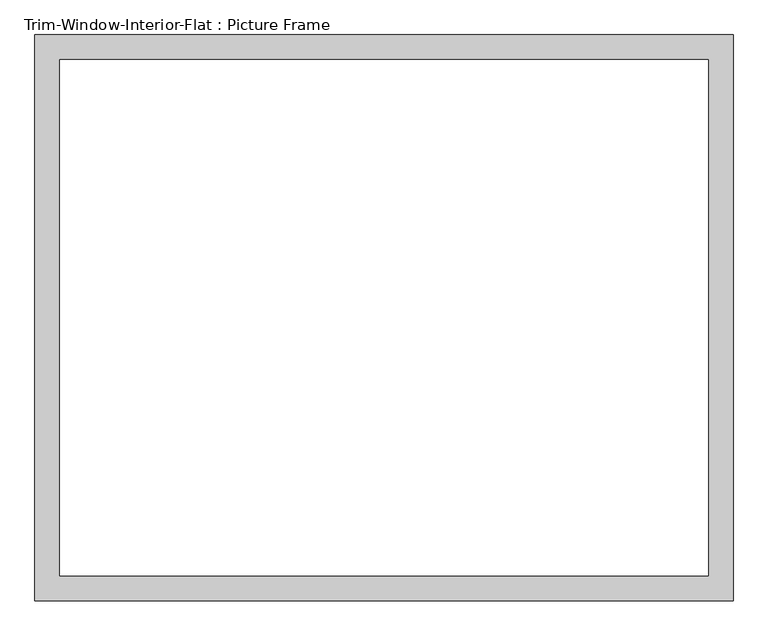
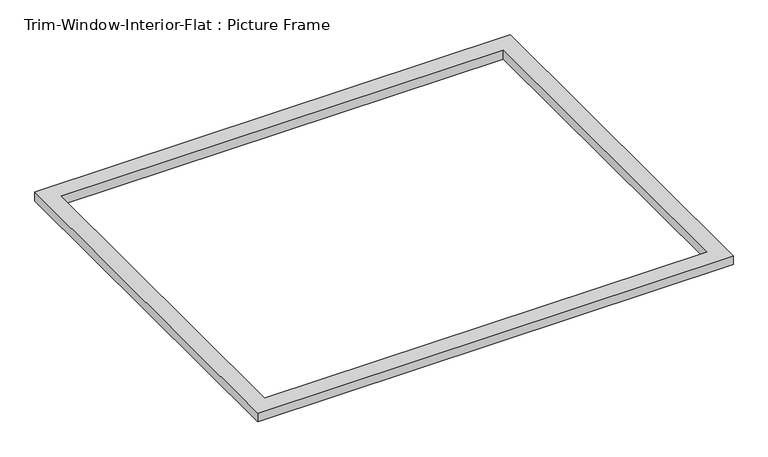
"""IFC4 building model written with IfcOpenShell, lengths in millimetres: proxy geometry, Trim-Window-Interior-Flat : Picture Frame."""

from ifc_helpers import new_model, si_unit, origin, origin_with_axes, place, context, project, spatial, polyline, outline, extrude, source, transform, mapped, element, save


def trim_window_interior_flat_picture_frame_0f2e31f9(model_context):
    return source(origin(), model_context, "Body", "SweptSolid", [
        extrude(outline(polyline([(806.45, 44.45), (806.45, -1263.65), (-806.45, -1263.65), (-806.45, 44.45), (806.45, 44.45)]), holes=[polyline([(749.3, -12.7), (-749.3, -12.7), (-749.3, -1206.5), (749.3, -1206.5), (749.3, -12.7)])]), origin_with_axes(), (0.0, 0.0, 1.0), 31.75),
    ])


if __name__ == "__main__":
    model = new_model("IFC4")
    model_context = context("Model", 3, world=origin())
    ifc_project = project(units=[si_unit("LENGTHUNIT", "METRE", prefix="MILLI")], contexts=[model_context])
    site = spatial("IfcSite", under=ifc_project)
    building = spatial("IfcBuilding", under=site)
    placement = place(None, origin())
    trim_window_interior_flat_picture_frame_shape = trim_window_interior_flat_picture_frame_0f2e31f9(model_context)
    element("IfcBuildingElementProxy", 1, Name="Trim-Window-Interior-Flat : Picture Frame", ObjectType="Trim-Window-Interior-Flat : Picture Frame", at=placement, inside=building, context=model_context, shape_type="MappedRepresentation", body=[
        mapped(trim_window_interior_flat_picture_frame_shape, transform((0.0, 0.0, 0.0), x_axis=(1.0, 0.0, 0.0), y_axis=(0.0, 1.0, 0.0), z_axis=(0.0, 0.0, 1.0))),
    ])
    save(model, "model.ifc")

# Revit data of these elements
# Type "Trim-Window-Interior-Flat : Picture Frame"
#   Trim Thickness_Picture Frame = 0' - 1 1/4"
#   Trim Width = 0' - 2 1/4"
#   Trim Thickness_with Sill = 0' - 0 3/4"
#   Sill Thickness = 0' - 1 1/4"
#   Opening Width [instance default] = 2' - 0"
#   Opening Height [instance default] = 3' - 0"
#   Default Elevation = 4' - 0"
#   Sill = no
#   Picture Frame = yes
#   Trim Material [instance default] = none
# Element 1 (IfcBuildingElementProxy, "Trim-Window-Interior-Flat : Picture Frame")
#   Opening Width = 5' - 0"
#   Opening Height = 4' - 0"
#   Trim Material = Wood - Stained
#   Materials on its faces: "Wood - Stained"
# Materials
#   "Wood - Stained": class "Wood", colour RGB 224 178 126, transparency 0, Cost = 0
